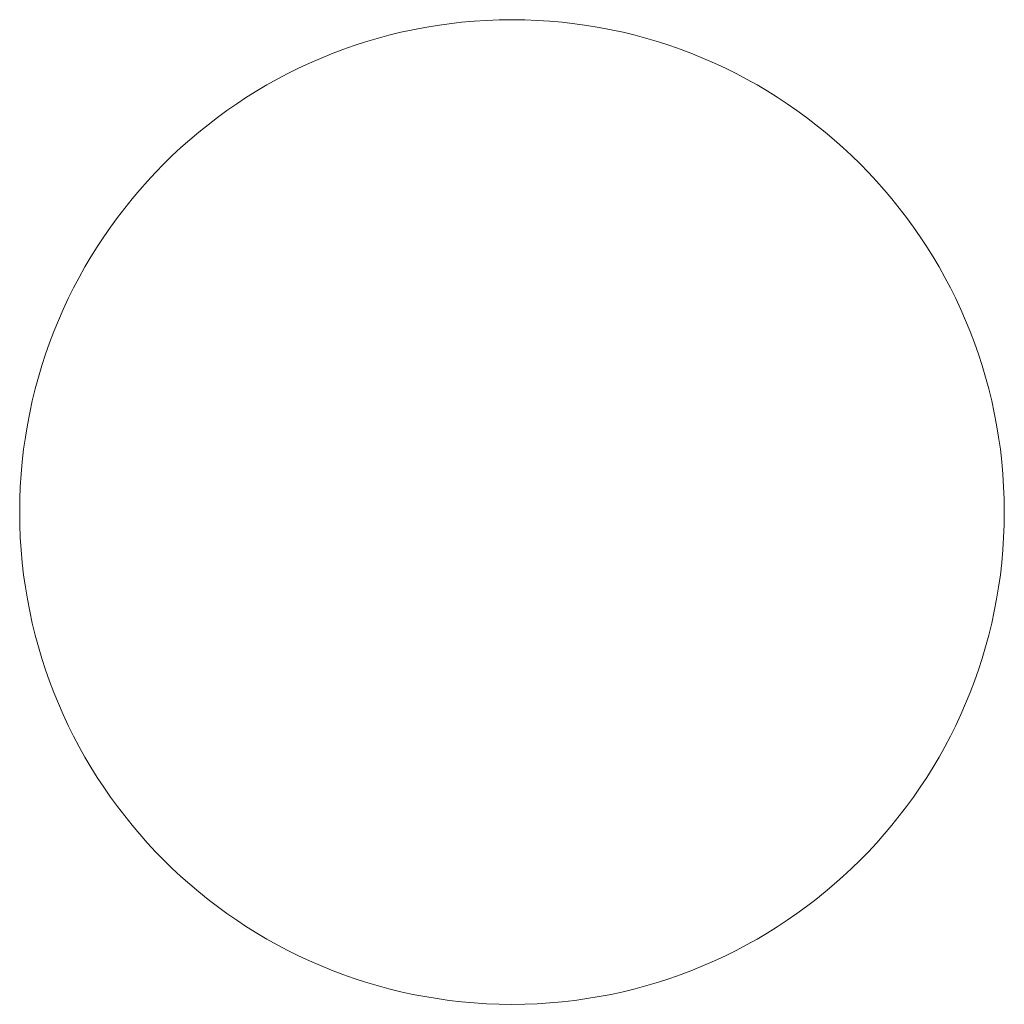
# Model space of a CAD drawing. Units: millimetres. Extents: x 755 to 878, y 1140 to 1263.
import ezdxf

# ---------------------------------------------------------------- set-up
doc = ezdxf.new("R2010")
doc.units = ezdxf.units.MM
doc.layers.add('M-CONS', color=8, linetype='Continuous', lineweight=18)

msp = doc.modelspace()

# ---------------------------------------------------------------- linework, layer by layer
at = {"layer": 'M-CONS'}
msp.add_circle((816.82, 1201.63, 22), 61.5, dxfattribs=at)

doc.saveas('drawing.dxf')
